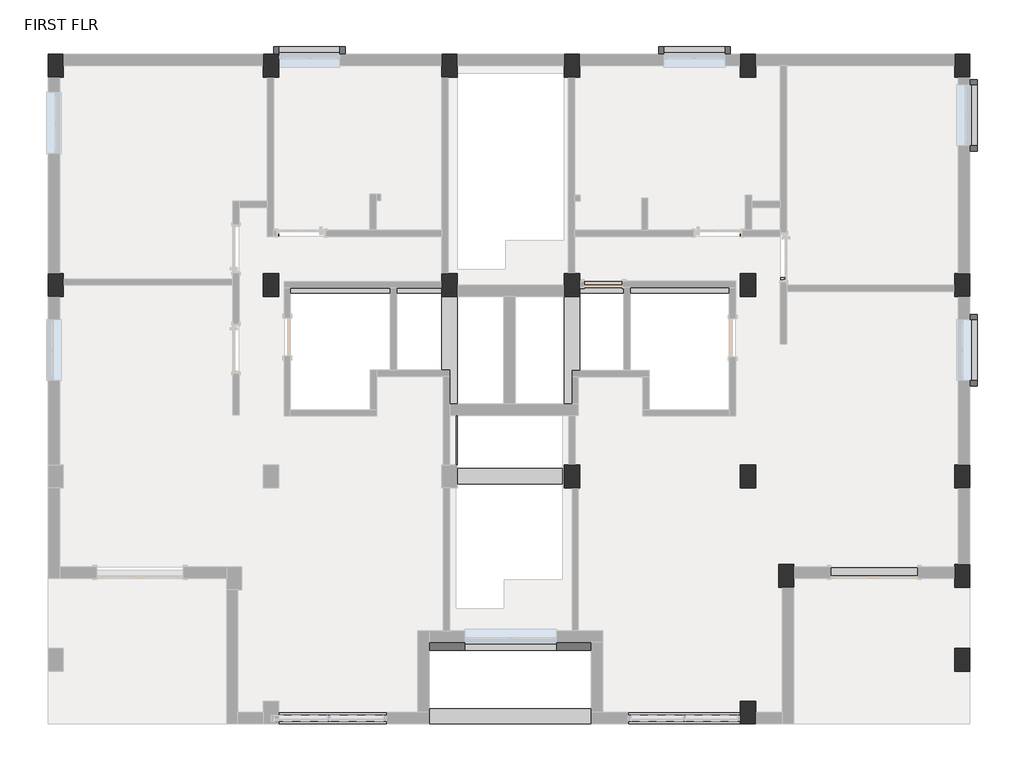
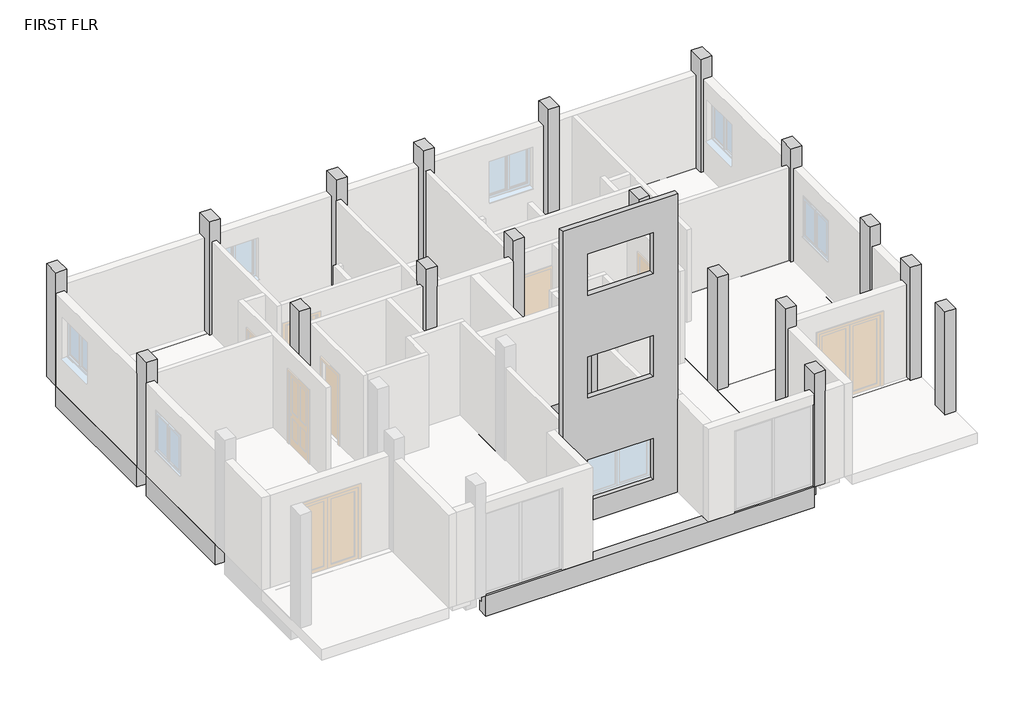
# One storey, part 3 of 3: 31 beams, 19 columns, 5 proxies, 1 light fixture.
"""IFC4 building model written with IfcOpenShell, lengths in millimetres."""

from ifc_helpers import new_model, si_unit, frame, origin, place, context, project, spatial, polyline, outline, extrude, faceted_brep, transform, mapped, element, save
from components import generic_models_10_generic_models_5_40bb8100, generic_models_13_generic_models_13_6edbfaa0, generic_models_2_generic_models_2_e2b5cfd4, column_11789f6a, family2_family2_8c2629c1

model = new_model("IFC4")

# Units and contexts
model_context = context("Model", 3, world=origin())
ifc_project = project(units=[si_unit("LENGTHUNIT", "METRE", prefix="MILLI")], contexts=[model_context])

# Site, building, storey
site = spatial("IfcSite", under=ifc_project)
building = spatial("IfcBuilding", under=site)
storey = spatial("IfcBuildingStorey", under=building, Name="FIRST FLR", Elevation=3352.8)

# Beams
placement = place(None, origin())
element("IfcBeam", 1, ObjectType="Concrete-Rectangular Beam : 12 x 24", at=placement, inside=storey, context=model_context, shape_type="SweptSolid", body=[
    extrude(outline(polyline([(-8839.9786397, -1604.6061634), (-8839.9786397, -1299.8061634), (-4852.9175798, -1299.8061634), (-4852.9175798, -1604.6061634), (-8839.9786397, -1604.6061634)])), frame((0.0, 0.0, 2743.2), z_axis=(0.0, 0.0, 1.0), x_axis=(1.0, 0.0, 0.0)), (0.0, 0.0, 1.0), 609.6),
])
element("IfcBeam", 2, ObjectType="Concrete-Rectangular Beam : 12 x 24", at=placement, inside=storey, context=model_context, shape_type="SweptSolid", body=[
    extrude(outline(polyline([(-1296.9175798, -1299.8061634), (-1296.9175798, -1604.6061634), (-4548.1175798, -1604.6061634), (-4548.1175798, -1299.8061634), (-1296.9175798, -1299.8061634)])), frame((0.0, 0.0, 2743.2), z_axis=(0.0, 0.0, 1.0), x_axis=(1.0, 0.0, 0.0)), (0.0, 0.0, 1.0), 609.6),
])
element("IfcBeam", 3, ObjectType="Concrete-Rectangular Beam : 12 x 24", at=placement, inside=storey, context=model_context, shape_type="SweptSolid", body=[
    extrude(outline(polyline([(1141.4824202, -1299.8061634), (1141.4824202, -1604.6061634), (-992.1175798, -1604.6061634), (-992.1175798, -1299.8061634), (1141.4824202, -1299.8061634)])), frame((0.0, 0.0, 2743.2), z_axis=(0.0, 0.0, 1.0), x_axis=(1.0, 0.0, 0.0)), (0.0, 0.0, 1.0), 609.6),
])
element("IfcBeam", 4, ObjectType="Concrete-Rectangular Beam : 12 x 24", at=placement, inside=storey, context=model_context, shape_type="SweptSolid", body=[
    extrude(outline(polyline([(4646.6824202, -1299.8061634), (4646.6824202, -1604.6061634), (1446.2824202, -1604.6061634), (1446.2824202, -1299.8061634), (4646.6824202, -1299.8061634)])), frame((0.0, 0.0, 2743.2), z_axis=(0.0, 0.0, 1.0), x_axis=(1.0, 0.0, 0.0)), (0.0, 0.0, 1.0), 609.6),
])
element("IfcBeam", 5, ObjectType="Concrete-Rectangular Beam : 12 x 24", at=placement, inside=storey, context=model_context, shape_type="SweptSolid", body=[
    extrude(outline(polyline([(8913.9345022, -1299.8061634), (8913.9345022, -1604.6061634), (4951.5345022, -1604.6061634), (4951.5345022, -1299.8061634), (8913.9345022, -1299.8061634)])), frame((0.0, 0.0, 2743.2), z_axis=(0.0, 0.0, 1.0), x_axis=(1.0, 0.0, 0.0)), (0.0, 0.0, 1.0), 609.6),
])
element("IfcBeam", 6, ObjectType="Concrete-Rectangular Beam : 12 x 24", at=placement, inside=storey, context=model_context, shape_type="SweptSolid", body=[
    extrude(outline(polyline([(9218.6824202, -5600.6620333), (8913.8824202, -5600.6620333), (8913.8824202, -1680.8061634), (9218.6824202, -1680.8061634), (9218.6824202, -5600.6620333)])), frame((0.0, 0.0, 2743.2), z_axis=(0.0, 0.0, 1.0), x_axis=(1.0, 0.0, 0.0)), (0.0, 0.0, 1.0), 609.6),
])
element("IfcBeam", 7, ObjectType="Concrete-Rectangular Beam : 12 x 24", at=placement, inside=storey, context=model_context, shape_type="SweptSolid", body=[
    extrude(outline(polyline([(9218.6824202, -9410.6620333), (8913.8824202, -9410.6620333), (8913.8824202, -6057.8620333), (9218.6824202, -6057.8620333), (9218.6824202, -9410.6620333)])), frame((0.0, 0.0, 2743.2), z_axis=(0.0, 0.0, 1.0), x_axis=(1.0, 0.0, 0.0)), (0.0, 0.0, 1.0), 609.6),
])
element("IfcBeam", 8, ObjectType="Concrete-Rectangular Beam : 12 x 24", at=placement, inside=storey, context=model_context, shape_type="SweptSolid", body=[
    extrude(outline(polyline([(9218.6824202, -11391.8620333), (8913.8824202, -11391.8620333), (8913.8824202, -9867.8620333), (9218.6824202, -9867.8620333), (9218.6824202, -11391.8620333)])), frame((0.0, 0.0, 2743.2), z_axis=(0.0, 0.0, 1.0), x_axis=(1.0, 0.0, 0.0)), (0.0, 0.0, 1.0), 609.6),
])
element("IfcBeam", 9, ObjectType="Concrete-Rectangular Beam : 12 x 24", at=placement, inside=storey, context=model_context, shape_type="SweptSolid", body=[
    extrude(outline(polyline([(-8839.9786397, -5600.6620333), (-9144.7786397, -5600.6620333), (-9144.7786397, -1680.8061634), (-8839.9786397, -1680.8061634), (-8839.9786397, -5600.6620333)])), frame((0.0, 0.0, 2743.2), z_axis=(0.0, 0.0, 1.0), x_axis=(1.0, 0.0, 0.0)), (0.0, 0.0, 1.0), 609.6),
])
element("IfcBeam", 10, ObjectType="Concrete-Rectangular Beam : 12 x 24", at=placement, inside=storey, context=model_context, shape_type="SweptSolid", body=[
    extrude(outline(polyline([(-8839.9786397, -9410.6620333), (-9144.7786397, -9410.6620333), (-9144.7786397, -6057.8620333), (-8839.9786397, -6057.8620333), (-8839.9786397, -9410.6620333)])), frame((0.0, 0.0, 2743.2), z_axis=(0.0, 0.0, 1.0), x_axis=(1.0, 0.0, 0.0)), (0.0, 0.0, 1.0), 609.6),
])
element("IfcBeam", 11, ObjectType="Concrete-Rectangular Beam : 12 x 24", at=placement, inside=storey, context=model_context, shape_type="SweptSolid", body=[
    extrude(outline(polyline([(4951.4824202, -5981.6620333), (4951.4824202, -5676.8620333), (8913.8824202, -5676.8620333), (8913.8824202, -5981.6620333), (4951.4824202, -5981.6620333)])), frame((0.0, 0.0, 2743.2), z_axis=(0.0, 0.0, 1.0), x_axis=(1.0, 0.0, 0.0)), (0.0, 0.0, 1.0), 609.6),
])
element("IfcBeam", 12, ObjectType="Concrete-Rectangular Beam : 12 x 24", at=placement, inside=storey, context=model_context, shape_type="SweptSolid", body=[
    extrude(outline(polyline([(1446.2824202, -5981.6620333), (1446.2824202, -5676.8620333), (4646.6824202, -5676.8620333), (4646.6824202, -5981.6620333), (1446.2824202, -5981.6620333)])), frame((0.0, 0.0, 2743.2), z_axis=(0.0, 0.0, 1.0), x_axis=(1.0, 0.0, 0.0)), (0.0, 0.0, 1.0), 609.6),
])
element("IfcBeam", 13, ObjectType="Concrete-Rectangular Beam : 12 x 24", at=placement, inside=storey, context=model_context, shape_type="SweptSolid", body=[
    extrude(outline(polyline([(-992.1175798, -5981.6620333), (-992.1175798, -5676.8620333), (1141.4824202, -5676.8620333), (1141.4824202, -5981.6620333), (-992.1175798, -5981.6620333)])), frame((0.0, 0.0, 2743.2), z_axis=(0.0, 0.0, 1.0), x_axis=(1.0, 0.0, 0.0)), (0.0, 0.0, 1.0), 609.6),
])
element("IfcBeam", 14, ObjectType="Concrete-Rectangular Beam : 12 x 24", at=placement, inside=storey, context=model_context, shape_type="SweptSolid", body=[
    extrude(outline(polyline([(-4548.1175798, -5981.6620333), (-4548.1175798, -5676.8620333), (-1296.9175798, -5676.8620333), (-1296.9175798, -5981.6620333), (-4548.1175798, -5981.6620333)])), frame((0.0, 0.0, 2743.2), z_axis=(0.0, 0.0, 1.0), x_axis=(1.0, 0.0, 0.0)), (0.0, 0.0, 1.0), 609.6),
])
element("IfcBeam", 15, ObjectType="Concrete-Rectangular Beam : 12 x 24", at=placement, inside=storey, context=model_context, shape_type="SweptSolid", body=[
    extrude(outline(polyline([(-8839.9786397, -5981.6620333), (-8839.9786397, -5676.8620333), (-4852.9175798, -5676.8620333), (-4852.9175798, -5981.6620333), (-8839.9786397, -5981.6620333)])), frame((0.0, 0.0, 2743.2), z_axis=(0.0, 0.0, 1.0), x_axis=(1.0, 0.0, 0.0)), (0.0, 0.0, 1.0), 609.6),
])
element("IfcBeam", 16, ObjectType="Concrete-Rectangular Beam : 12 x 24", at=placement, inside=storey, context=model_context, shape_type="SweptSolid", body=[
    extrude(outline(polyline([(1446.2824202, -9791.6620333), (1446.2824202, -9486.8620333), (4646.6824202, -9486.8620333), (4646.6824202, -9791.6620333), (1446.2824202, -9791.6620333)])), frame((0.0, 0.0, 2743.2), z_axis=(0.0, 0.0, 1.0), x_axis=(1.0, 0.0, 0.0)), (0.0, 0.0, 1.0), 609.6),
])
element("IfcBeam", 17, ObjectType="Concrete-Rectangular Beam : 12 x 24", at=placement, inside=storey, context=model_context, shape_type="Brep", body=[
    faceted_brep([(4951.4824202, -9867.8620333, 3352.8), (4646.6824202, -9867.8620333, 3352.8), (4646.6824202, -11772.8620333, 3352.8), (4951.4824202, -11772.8620333, 3352.8), (4951.4824202, -11468.0620333, 3352.8), (4646.6824202, -9867.8620333, 2743.2), (4646.6824202, -11772.8620333, 2743.2), (4951.4824202, -9867.8620333, 2743.2), (4951.4824202, -11468.0620333, 2743.2), (4951.4824202, -11772.8620333, 2743.2)], [[[0, 1, 2, 3, 4]], [[1, 5, 6, 2]], [[5, 7, 8, 9, 6]], [[7, 0, 4, 3, 9, 8]], [[0, 7, 5, 1]], [[3, 2, 6, 9]]]),
])
element("IfcBeam", 18, ObjectType="Concrete-Rectangular Beam : 12 x 24", at=placement, inside=storey, context=model_context, shape_type="SweptSolid", body=[
    extrude(outline(polyline([(5408.6824202, -11468.0620333), (5408.6824202, -11772.8620333), (4951.4824202, -11772.8620333), (4951.4824202, -11468.0620333), (5408.6824202, -11468.0620333)])), frame((0.0, 0.0, 2743.2), z_axis=(0.0, 0.0, 1.0), x_axis=(1.0, 0.0, 0.0)), (0.0, 0.0, 1.0), 609.6),
])
element("IfcBeam", 19, ObjectType="Concrete-Rectangular Beam : 12 x 24", at=placement, inside=storey, context=model_context, shape_type="SweptSolid", body=[
    extrude(outline(polyline([(8913.8824202, -11468.0620333), (8913.8824202, -11772.8620333), (5713.4824202, -11772.8620333), (5713.4824202, -11468.0620333), (8913.8824202, -11468.0620333)])), frame((0.0, 0.0, 2743.2), z_axis=(0.0, 0.0, 1.0), x_axis=(1.0, 0.0, 0.0)), (0.0, 0.0, 1.0), 609.6),
])
element("IfcBeam", 20, ObjectType="Concrete-Rectangular Beam : 12 x 24", at=placement, inside=storey, context=model_context, shape_type="SweptSolid", body=[
    extrude(outline(polyline([(4646.6824202, -14272.0402089), (4646.6824202, -14576.8402089), (-4548.1175798, -14576.8402089), (-4548.1175798, -14272.0402089), (4646.6824202, -14272.0402089)])), frame((0.0, 0.0, 2743.2), z_axis=(0.0, 0.0, 1.0), x_axis=(1.0, 0.0, 0.0)), (0.0, 0.0, 1.0), 609.6),
])
element("IfcBeam", 21, ObjectType="Concrete-Rectangular Beam : 12 x 24", at=placement, inside=storey, context=model_context, shape_type="SweptSolid", body=[
    extrude(outline(polyline([(4951.4824202, -14119.6402089), (4646.6824202, -14119.6402089), (4646.6824202, -11772.8620333), (4951.4824202, -11772.8620333), (4951.4824202, -14119.6402089)])), frame((0.0, 0.0, 2743.2), z_axis=(0.0, 0.0, 1.0), x_axis=(1.0, 0.0, 0.0)), (0.0, 0.0, 1.0), 609.6),
])
element("IfcBeam", 22, ObjectType="Concrete-Rectangular Beam : 12 x 24", at=placement, inside=storey, context=model_context, shape_type="SweptSolid", body=[
    extrude(outline(polyline([(-4548.1175798, -5600.6620333), (-4852.9175798, -5600.6620333), (-4852.9175798, -1680.8061634), (-4548.1175798, -1680.8061634), (-4548.1175798, -5600.6620333)])), frame((0.0, 0.0, 2743.2), z_axis=(0.0, 0.0, 1.0), x_axis=(1.0, 0.0, 0.0)), (0.0, 0.0, 1.0), 609.6),
])
element("IfcBeam", 23, ObjectType="Concrete-Rectangular Beam : 12 x 24", at=placement, inside=storey, context=model_context, shape_type="SweptSolid", body=[
    extrude(outline(polyline([(-4548.1175798, -9410.6620333), (-4852.9175798, -9410.6620333), (-4852.9175798, -6057.8620333), (-4548.1175798, -6057.8620333), (-4548.1175798, -9410.6620333)])), frame((0.0, 0.0, 2743.2), z_axis=(0.0, 0.0, 1.0), x_axis=(1.0, 0.0, 0.0)), (0.0, 0.0, 1.0), 609.6),
])
element("IfcBeam", 24, ObjectType="Concrete-Rectangular Beam : 12 x 24", at=placement, inside=storey, context=model_context, shape_type="SweptSolid", body=[
    extrude(outline(polyline([(-992.1175798, -5600.6620333), (-1296.9175798, -5600.6620333), (-1296.9175798, -1680.8061634), (-992.1175798, -1680.8061634), (-992.1175798, -5600.6620333)])), frame((0.0, 0.0, 2743.2), z_axis=(0.0, 0.0, 1.0), x_axis=(1.0, 0.0, 0.0)), (0.0, 0.0, 1.0), 609.6),
])
element("IfcBeam", 25, ObjectType="Concrete-Rectangular Beam : 12 x 24", at=placement, inside=storey, context=model_context, shape_type="SweptSolid", body=[
    extrude(outline(polyline([(-992.1175798, -9410.6620333), (-1296.9175798, -9410.6620333), (-1296.9175798, -6057.8620333), (-992.1175798, -6057.8620333), (-992.1175798, -9410.6620333)])), frame((0.0, 0.0, 2743.2), z_axis=(0.0, 0.0, 1.0), x_axis=(1.0, 0.0, 0.0)), (0.0, 0.0, 1.0), 609.6),
])
element("IfcBeam", 26, ObjectType="Concrete-Rectangular Beam : 12 x 24", at=placement, inside=storey, context=model_context, shape_type="SweptSolid", body=[
    extrude(outline(polyline([(1141.4824202, -6057.8620333), (1446.2824202, -6057.8620333), (1446.2824202, -9410.6620333), (1141.4824202, -9410.6620333), (1141.4824202, -6057.8620333)])), frame((0.0, 0.0, 2743.2), z_axis=(0.0, 0.0, 1.0), x_axis=(1.0, 0.0, 0.0)), (0.0, 0.0, 1.0), 609.6),
])
element("IfcBeam", 27, ObjectType="Concrete-Rectangular Beam : 12 x 24", at=placement, inside=storey, context=model_context, shape_type="SweptSolid", body=[
    extrude(outline(polyline([(1141.4824202, -1680.8061634), (1446.2824202, -1680.8061634), (1446.2824202, -5600.6620333), (1141.4824202, -5600.6620333), (1141.4824202, -1680.8061634)])), frame((0.0, 0.0, 2743.2), z_axis=(0.0, 0.0, 1.0), x_axis=(1.0, 0.0, 0.0)), (0.0, 0.0, 1.0), 609.6),
])
element("IfcBeam", 28, ObjectType="Concrete-Rectangular Beam : 12 x 24", at=placement, inside=storey, context=model_context, shape_type="SweptSolid", body=[
    extrude(outline(polyline([(4951.4824202, -5600.6620333), (4646.6824202, -5600.6620333), (4646.6824202, -1680.8061634), (4951.4824202, -1680.8061634), (4951.4824202, -5600.6620333)])), frame((0.0, 0.0, 2743.2), z_axis=(0.0, 0.0, 1.0), x_axis=(1.0, 0.0, 0.0)), (0.0, 0.0, 1.0), 609.6),
])
element("IfcBeam", 29, ObjectType="Concrete-Rectangular Beam : 12 x 24", at=placement, inside=storey, context=model_context, shape_type="SweptSolid", body=[
    extrude(outline(polyline([(4951.4824202, -9410.6620333), (4646.6824202, -9410.6620333), (4646.6824202, -6057.8620333), (4951.4824202, -6057.8620333), (4951.4824202, -9410.6620333)])), frame((0.0, 0.0, 2743.2), z_axis=(0.0, 0.0, 1.0), x_axis=(1.0, 0.0, 0.0)), (0.0, 0.0, 1.0), 609.6),
])
element("IfcBeam", 30, ObjectType="Concrete-Rectangular Beam : 12 x 24", at=placement, inside=storey, context=model_context, shape_type="SweptSolid", body=[
    extrude(outline(polyline([(4951.4824202, -9791.6620333), (4951.4824202, -9486.8620333), (8913.8824202, -9486.8620333), (8913.8824202, -9791.6620333), (4951.4824202, -9791.6620333)])), frame((0.0, 0.0, 2743.2), z_axis=(0.0, 0.0, 1.0), x_axis=(1.0, 0.0, 0.0)), (0.0, 0.0, 1.0), 609.6),
])
element("IfcBeam", 31, ObjectType="Concrete-Rectangular Beam : 12 x 24", at=placement, inside=storey, context=model_context, shape_type="SweptSolid", body=[
    extrude(outline(polyline([(1141.4824202, -9486.8620333), (1141.4824202, -9791.6620333), (-992.1175798, -9791.6620333), (-992.1175798, -9486.8620333), (1141.4824202, -9486.8620333)])), frame((0.0, 0.0, 2743.2), z_axis=(0.0, 0.0, 1.0), x_axis=(1.0, 0.0, 0.0)), (0.0, 0.0, 1.0), 609.6),
])

# Proxies
generic_models_10_generic_models_5_shape = generic_models_10_generic_models_5_40bb8100(model_context)
element("IfcBuildingElementProxy", 32, Name="Generic Models 11 : Generic Models 5", ObjectType="Generic Models 11 : Generic Models 5", at=placement, inside=storey, context=model_context, shape_type="MappedRepresentation", body=[
    mapped(generic_models_10_generic_models_5_shape, transform((0.0, 0.0, -6096.0), x_axis=(1.0, 0.0, 0.0), y_axis=(0.0, 1.0, 0.0), z_axis=(0.0, 0.0, 1.0))),
])
generic_models_13_generic_models_13_shape = generic_models_13_generic_models_13_6edbfaa0(model_context)
element("IfcBuildingElementProxy", 33, Name="Generic Models 16 : Generic Models 13", ObjectType="Generic Models 16 : Generic Models 13", at=placement, inside=storey, context=model_context, shape_type="MappedRepresentation", body=[
    mapped(generic_models_13_generic_models_13_shape, transform((0.0, 0.0, -6096.0), x_axis=(1.0, 0.0, 0.0), y_axis=(0.0, 1.0, 0.0), z_axis=(0.0, 0.0, 1.0))),
])
element("IfcBuildingElementProxy", 34, Name="Generic Models 17 : Generic Models 13", ObjectType="Generic Models 17 : Generic Models 13", at=placement, inside=storey, context=model_context, shape_type="MappedRepresentation", body=[
    mapped(generic_models_13_generic_models_13_shape, transform((-7670.8, 0.0, -6096.0), x_axis=(1.0, 0.0, 0.0), y_axis=(0.0, 1.0, 0.0), z_axis=(0.0, 0.0, 1.0))),
])
generic_models_2_generic_models_2_shape = generic_models_2_generic_models_2_e2b5cfd4(model_context)
element("IfcBuildingElementProxy", 35, Name="Generic Models 2 : Generic Models 2", ObjectType="Generic Models 2 : Generic Models 2", at=placement, inside=storey, context=model_context, shape_type="MappedRepresentation", body=[
    mapped(generic_models_2_generic_models_2_shape, transform((0.0, 0.0, 0.0), x_axis=(1.0, 0.0, 0.0), y_axis=(0.0, 1.0, 0.0), z_axis=(0.0, 0.0, 1.0))),
])
element("IfcBuildingElementProxy", 36, Name="Generic Models 8 : Generic Models 5", ObjectType="Generic Models 8 : Generic Models 5", at=placement, inside=storey, context=model_context, shape_type="MappedRepresentation", body=[
    mapped(generic_models_10_generic_models_5_shape, transform((0.0, 4681.8558699, -6096.0), x_axis=(1.0, 0.0, 0.0), y_axis=(0.0, 1.0, 0.0), z_axis=(0.0, 0.0, 1.0))),
])

# Columns
element("IfcColumn", 37, ObjectType="Concrete-Rectangular-Column : 1'6\" X 1' COLUMN", at=placement, inside=storey, context=model_context, shape_type="Brep", body=[
    faceted_brep([(-8839.9786397, -1223.6061634, 3352.8), (-8839.9786397, -1680.8061634, 3352.8), (-9144.7786397, -1680.8061634, 3352.8), (-9144.7786397, -1223.6061634, 3352.8), (-8839.9786397, -1223.6061634, 6705.6), (-8839.9786397, -1299.8061634, 6705.6), (-8839.9786397, -1604.6061634, 6705.6), (-8839.9786397, -1680.8061634, 6705.6), (-8839.9786397, -1680.8061634, 6096.0), (-8839.9786397, -1680.8061634, 5791.2), (-9144.7786397, -1680.8061634, 6705.6), (-9144.7786397, -1680.8061634, 6096.0), (-9144.7786397, -1680.8061634, 5791.2), (-9144.7786397, -1223.6061634, 6705.6)], [[[0, 1, 2, 3]], [[4, 5, 6, 7, 8, 9, 1, 0]], [[7, 10, 11, 12, 2, 1, 9, 8]], [[10, 13, 3, 2, 12, 11]], [[13, 4, 0, 3]], [[4, 13, 10, 7, 6, 5]]]),
])
element("IfcColumn", 38, ObjectType="Concrete-Rectangular-Column : 1'6\" X 1' COLUMN", at=placement, inside=storey, context=model_context, shape_type="Brep", body=[
    faceted_brep([(-4548.1175798, -1223.6061634, 3352.8), (-4548.1175798, -1680.8061634, 3352.8), (-4852.9175798, -1680.8061634, 3352.8), (-4852.9175798, -1223.6061634, 3352.8), (-4548.1175798, -1223.6061634, 6705.6), (-4548.1175798, -1299.8061634, 6705.6), (-4548.1175798, -1604.6061634, 6705.6), (-4548.1175798, -1680.8061634, 6705.6), (-4548.1175798, -1680.8061634, 6096.0), (-4548.1175798, -1680.8061634, 5791.2), (-4852.9175798, -1680.8061634, 6705.6), (-4852.9175798, -1680.8061634, 6096.0), (-4852.9175798, -1680.8061634, 5791.2), (-4852.9175798, -1223.6061634, 6705.6)], [[[0, 1, 2, 3]], [[4, 5, 6, 7, 8, 9, 1, 0]], [[7, 10, 11, 12, 2, 1, 9, 8]], [[10, 13, 3, 2, 12, 11]], [[13, 4, 0, 3]], [[4, 13, 10, 7, 6, 5]]]),
])
element("IfcColumn", 39, ObjectType="Concrete-Rectangular-Column : 1'6\" X 1' COLUMN", at=placement, inside=storey, context=model_context, shape_type="Brep", body=[
    faceted_brep([(-992.1175798, -1223.6061634, 3352.8), (-992.1175798, -1680.8061634, 3352.8), (-1296.9175798, -1680.8061634, 3352.8), (-1296.9175798, -1223.6061634, 3352.8), (-992.1175798, -1223.6061634, 6705.6), (-992.1175798, -1299.8061634, 6705.6), (-992.1175798, -1604.6061634, 6705.6), (-992.1175798, -1680.8061634, 6705.6), (-992.1175798, -1680.8061634, 6096.0), (-992.1175798, -1680.8061634, 5791.2), (-1296.9175798, -1680.8061634, 6705.6), (-1296.9175798, -1680.8061634, 6096.0), (-1296.9175798, -1680.8061634, 5791.2), (-1296.9175798, -1604.6061634, 6705.6), (-1296.9175798, -1299.8061634, 6705.6), (-1296.9175798, -1223.6061634, 6705.6)], [[[0, 1, 2, 3]], [[4, 5, 6, 7, 8, 9, 1, 0]], [[7, 10, 11, 12, 2, 1, 9, 8]], [[10, 13, 14, 15, 3, 2, 12, 11]], [[15, 4, 0, 3]], [[4, 15, 14, 13, 10, 7, 6, 5]]]),
])
element("IfcColumn", 40, ObjectType="Concrete-Rectangular-Column : 1'6\" X 1' COLUMN", at=placement, inside=storey, context=model_context, shape_type="Brep", body=[
    faceted_brep([(1446.2824202, -1223.6061634, 3352.8), (1446.2824202, -1680.8061634, 3352.8), (1141.4824202, -1680.8061634, 3352.8), (1141.4824202, -1223.6061634, 3352.8), (1446.2824202, -1223.6061634, 6705.6), (1446.2824202, -1299.8061634, 6705.6), (1446.2824202, -1604.6061634, 6705.6), (1446.2824202, -1680.8061634, 6705.6), (1446.2824202, -1680.8061634, 6096.0), (1446.2824202, -1680.8061634, 5791.2), (1141.4824202, -1680.8061634, 6705.6), (1141.4824202, -1680.8061634, 6096.0), (1141.4824202, -1680.8061634, 5791.2), (1141.4824202, -1604.6061634, 6705.6), (1141.4824202, -1299.8061634, 6705.6), (1141.4824202, -1223.6061634, 6705.6)], [[[0, 1, 2, 3]], [[4, 5, 6, 7, 8, 9, 1, 0]], [[7, 10, 11, 12, 2, 1, 9, 8]], [[10, 13, 14, 15, 3, 2, 12, 11]], [[15, 4, 0, 3]], [[4, 15, 14, 13, 10, 7, 6, 5]]]),
])
element("IfcColumn", 41, ObjectType="Concrete-Rectangular-Column : 1'6\" X 1' COLUMN", at=placement, inside=storey, context=model_context, shape_type="Brep", body=[
    faceted_brep([(4951.4824202, -1223.6061634, 3352.8), (4951.4824202, -1680.8061634, 3352.8), (4646.6824202, -1680.8061634, 3352.8), (4646.6824202, -1223.6061634, 3352.8), (4951.4824202, -1223.6061634, 6705.6), (4951.4824202, -1680.8061634, 6705.6), (4951.4824202, -1680.8061634, 6096.0), (4951.4824202, -1680.8061634, 5791.2), (4646.6824202, -1680.8061634, 6705.6), (4646.6824202, -1680.8061634, 6096.0), (4646.6824202, -1680.8061634, 5791.2), (4646.6824202, -1604.6061634, 6705.6), (4646.6824202, -1299.8061634, 6705.6), (4646.6824202, -1223.6061634, 6705.6)], [[[0, 1, 2, 3]], [[4, 5, 6, 7, 1, 0]], [[5, 8, 9, 10, 2, 1, 7, 6]], [[8, 11, 12, 13, 3, 2, 10, 9]], [[13, 4, 0, 3]], [[4, 13, 12, 11, 8, 5]]]),
])
element("IfcColumn", 42, ObjectType="Concrete-Rectangular-Column : 1'6\" X 1' COLUMN", at=placement, inside=storey, context=model_context, shape_type="Brep", body=[
    faceted_brep([(9218.6824202, -1223.6061634, 3352.8), (9218.6824202, -1680.8061634, 3352.8), (8913.8824202, -1680.8061634, 3352.8), (8913.8824202, -1223.6061634, 3352.8), (9218.6824202, -1223.6061634, 6705.6), (9218.6824202, -1680.8061634, 6705.6), (9218.6824202, -1680.8061634, 6096.0), (9218.6824202, -1680.8061634, 5791.2), (8913.8824202, -1680.8061634, 6705.6), (8913.8824202, -1680.8061634, 6096.0), (8913.8824202, -1680.8061634, 5791.2), (8913.8824202, -1223.6061634, 6705.6)], [[[0, 1, 2, 3]], [[4, 5, 6, 7, 1, 0]], [[5, 8, 9, 10, 2, 1, 7, 6]], [[8, 11, 3, 2, 10, 9]], [[11, 4, 0, 3]], [[4, 11, 8, 5]]]),
])
element("IfcColumn", 43, ObjectType="Concrete-Rectangular-Column : 1'6\" X 1' COLUMN", at=placement, inside=storey, context=model_context, shape_type="Brep", body=[
    faceted_brep([(9218.6824202, -5600.6620333, 3352.8), (9218.6824202, -6057.8620333, 3352.8), (8913.8824202, -6057.8620333, 3352.8), (8913.8824202, -5600.6620333, 3352.8), (9218.6824202, -5600.6620333, 6705.6), (9218.6824202, -6057.8620333, 6705.6), (9218.6824202, -6057.8620333, 6096.0), (9218.6824202, -6057.8620333, 5791.2), (9218.6824202, -5600.6620333, 5791.2), (9218.6824202, -5600.6620333, 6096.0), (8913.8824202, -6057.8620333, 6705.6), (8913.8824202, -6057.8620333, 6096.0), (8913.8824202, -6057.8620333, 5791.2), (8913.8824202, -5981.6620333, 6705.6), (8913.8824202, -5676.8620333, 6705.6), (8913.8824202, -5600.6620333, 6705.6), (8913.8824202, -5600.6620333, 6096.0), (8913.8824202, -5600.6620333, 5791.2)], [[[0, 1, 2, 3]], [[4, 5, 6, 7, 1, 0, 8, 9]], [[5, 10, 11, 12, 2, 1, 7, 6]], [[10, 13, 14, 15, 16, 17, 3, 2, 12, 11]], [[15, 4, 9, 8, 0, 3, 17, 16]], [[4, 15, 14, 13, 10, 5]]]),
])
element("IfcColumn", 44, ObjectType="Concrete-Rectangular-Column : 1'6\" X 1' COLUMN", at=placement, inside=storey, context=model_context, shape_type="Brep", body=[
    faceted_brep([(4951.4824202, -5600.6620333, 3352.8), (4951.4824202, -6057.8620333, 3352.8), (4646.6824202, -6057.8620333, 3352.8), (4646.6824202, -5600.6620333, 3352.8), (4951.4824202, -5600.6620333, 6705.6), (4951.4824202, -5676.8620333, 6705.6), (4951.4824202, -5981.6620333, 6705.6), (4951.4824202, -6057.8620333, 6705.6), (4951.4824202, -6057.8620333, 6096.0), (4951.4824202, -6057.8620333, 5791.2), (4951.4824202, -5600.6620333, 5791.2), (4951.4824202, -5600.6620333, 6096.0), (4646.6824202, -6057.8620333, 6705.6), (4646.6824202, -6057.8620333, 6096.0), (4646.6824202, -6057.8620333, 5791.2), (4646.6824202, -5981.6620333, 6705.6), (4646.6824202, -5676.8620333, 6705.6), (4646.6824202, -5600.6620333, 6705.6), (4646.6824202, -5600.6620333, 6096.0), (4646.6824202, -5600.6620333, 5791.2)], [[[0, 1, 2, 3]], [[4, 5, 6, 7, 8, 9, 1, 0, 10, 11]], [[7, 12, 13, 14, 2, 1, 9, 8]], [[12, 15, 16, 17, 18, 19, 3, 2, 14, 13]], [[17, 4, 11, 10, 0, 3, 19, 18]], [[4, 17, 16, 15, 12, 7, 6, 5]]]),
])
element("IfcColumn", 45, ObjectType="Concrete-Rectangular-Column : 1'6\" X 1' COLUMN", at=placement, inside=storey, context=model_context, shape_type="Brep", body=[
    faceted_brep([(1446.2824202, -5600.6620333, 3352.8), (1446.2824202, -6057.8620333, 3352.8), (1141.4824202, -6057.8620333, 3352.8), (1141.4824202, -5600.6620333, 3352.8), (1446.2824202, -5600.6620333, 6705.6), (1446.2824202, -5676.8620333, 6705.6), (1446.2824202, -5981.6620333, 6705.6), (1446.2824202, -6057.8620333, 6705.6), (1446.2824202, -6057.8620333, 6096.0), (1446.2824202, -6057.8620333, 5791.2), (1446.2824202, -5600.6620333, 5791.2), (1446.2824202, -5600.6620333, 6096.0), (1141.4824202, -6057.8620333, 6705.6), (1141.4824202, -6057.8620333, 6096.0), (1141.4824202, -6057.8620333, 5791.2), (1141.4824202, -5981.6620333, 6705.6), (1141.4824202, -5676.8620333, 6705.6), (1141.4824202, -5600.6620333, 6705.6), (1141.4824202, -5600.6620333, 6096.0), (1141.4824202, -5600.6620333, 5791.2)], [[[0, 1, 2, 3]], [[4, 5, 6, 7, 8, 9, 1, 0, 10, 11]], [[7, 12, 13, 14, 2, 1, 9, 8]], [[12, 15, 16, 17, 18, 19, 3, 2, 14, 13]], [[17, 4, 11, 10, 0, 3, 19, 18]], [[4, 17, 16, 15, 12, 7, 6, 5]]]),
])
element("IfcColumn", 46, ObjectType="Concrete-Rectangular-Column : 1'6\" X 1' COLUMN", at=placement, inside=storey, context=model_context, shape_type="Brep", body=[
    faceted_brep([(-992.1175798, -5600.6620333, 3352.8), (-992.1175798, -6057.8620333, 3352.8), (-1296.9175798, -6057.8620333, 3352.8), (-1296.9175798, -5600.6620333, 3352.8), (-992.1175798, -5600.6620333, 6705.6), (-992.1175798, -5676.8620333, 6705.6), (-992.1175798, -5981.6620333, 6705.6), (-992.1175798, -6057.8620333, 6705.6), (-992.1175798, -6057.8620333, 6096.0), (-992.1175798, -6057.8620333, 5791.2), (-992.1175798, -5600.6620333, 5791.2), (-992.1175798, -5600.6620333, 6096.0), (-1296.9175798, -6057.8620333, 6705.6), (-1296.9175798, -6057.8620333, 6096.0), (-1296.9175798, -6057.8620333, 5791.2), (-1296.9175798, -5981.6620333, 6705.6), (-1296.9175798, -5676.8620333, 6705.6), (-1296.9175798, -5600.6620333, 6705.6), (-1296.9175798, -5600.6620333, 6096.0), (-1296.9175798, -5600.6620333, 5791.2)], [[[0, 1, 2, 3]], [[4, 5, 6, 7, 8, 9, 1, 0, 10, 11]], [[7, 12, 13, 14, 2, 1, 9, 8]], [[12, 15, 16, 17, 18, 19, 3, 2, 14, 13]], [[17, 4, 11, 10, 0, 3, 19, 18]], [[4, 17, 16, 15, 12, 7, 6, 5]]]),
])
element("IfcColumn", 47, ObjectType="Concrete-Rectangular-Column : 1'6\" X 1' COLUMN", at=placement, inside=storey, context=model_context, shape_type="Brep", body=[
    faceted_brep([(-4548.1175798, -5600.6620333, 3352.8), (-4548.1175798, -6057.8620333, 3352.8), (-4852.9175798, -6057.8620333, 3352.8), (-4852.9175798, -5600.6620333, 3352.8), (-4548.1175798, -5600.6620333, 6705.6), (-4548.1175798, -5676.8620333, 6705.6), (-4548.1175798, -5981.6620333, 6705.6), (-4548.1175798, -6057.8620333, 6705.6), (-4548.1175798, -6057.8620333, 6096.0), (-4548.1175798, -6057.8620333, 5791.2), (-4548.1175798, -5600.6620333, 5791.2), (-4548.1175798, -5600.6620333, 6096.0), (-4852.9175798, -6057.8620333, 6705.6), (-4852.9175798, -6057.8620333, 6096.0), (-4852.9175798, -6057.8620333, 5791.2), (-4852.9175798, -5981.6620333, 6705.6), (-4852.9175798, -5676.8620333, 6705.6), (-4852.9175798, -5600.6620333, 6705.6), (-4852.9175798, -5600.6620333, 6096.0), (-4852.9175798, -5600.6620333, 5791.2)], [[[0, 1, 2, 3]], [[4, 5, 6, 7, 8, 9, 1, 0, 10, 11]], [[7, 12, 13, 14, 2, 1, 9, 8]], [[12, 15, 16, 17, 18, 19, 3, 2, 14, 13]], [[17, 4, 11, 10, 0, 3, 19, 18]], [[4, 17, 16, 15, 12, 7, 6, 5]]]),
])
element("IfcColumn", 48, ObjectType="Concrete-Rectangular-Column : 1'6\" X 1' COLUMN", at=placement, inside=storey, context=model_context, shape_type="Brep", body=[
    faceted_brep([(-8839.9786397, -5600.6620333, 3352.8), (-8839.9786397, -6057.8620333, 3352.8), (-9144.7786397, -6057.8620333, 3352.8), (-9144.7786397, -5600.6620333, 3352.8), (-8839.9786397, -5600.6620333, 6705.6), (-8839.9786397, -5676.8620333, 6705.6), (-8839.9786397, -5981.6620333, 6705.6), (-8839.9786397, -6057.8620333, 6705.6), (-8839.9786397, -6057.8620333, 6096.0), (-8839.9786397, -6057.8620333, 5791.2), (-8839.9786397, -5600.6620333, 5791.2), (-8839.9786397, -5600.6620333, 6096.0), (-9144.7786397, -6057.8620333, 6705.6), (-9144.7786397, -6057.8620333, 6096.0), (-9144.7786397, -6057.8620333, 5791.2), (-9144.7786397, -5600.6620333, 6705.6), (-9144.7786397, -5600.6620333, 6096.0), (-9144.7786397, -5600.6620333, 5791.2)], [[[0, 1, 2, 3]], [[4, 5, 6, 7, 8, 9, 1, 0, 10, 11]], [[7, 12, 13, 14, 2, 1, 9, 8]], [[12, 15, 16, 17, 3, 2, 14, 13]], [[15, 4, 11, 10, 0, 3, 17, 16]], [[4, 15, 12, 7, 6, 5]]]),
])
element("IfcColumn", 49, ObjectType="Concrete-Rectangular-Column : 1'6\" X 1' COLUMN", at=placement, inside=storey, context=model_context, shape_type="Brep", body=[
    faceted_brep([(9218.6824202, -11391.8620333, 3352.8), (9218.6824202, -11849.0620333, 3352.8), (8913.8824202, -11849.0620333, 3352.8), (8913.8824202, -11391.8620333, 3352.8), (9218.6824202, -11391.8620333, 6705.6), (9218.6824202, -11849.0620333, 6705.6), (9218.6824202, -11391.8620333, 5791.2), (9218.6824202, -11391.8620333, 6096.0), (8913.8824202, -11849.0620333, 6705.6), (8913.8824202, -11772.8620333, 6705.6), (8913.8824202, -11468.0620333, 6705.6), (8913.8824202, -11391.8620333, 6705.6), (8913.8824202, -11391.8620333, 6096.0), (8913.8824202, -11391.8620333, 5791.2)], [[[0, 1, 2, 3]], [[4, 5, 1, 0, 6, 7]], [[5, 8, 2, 1]], [[8, 9, 10, 11, 12, 13, 3, 2]], [[11, 4, 7, 6, 0, 3, 13, 12]], [[4, 11, 10, 9, 8, 5]]]),
])
element("IfcColumn", 50, ObjectType="Concrete-Rectangular-Column : 1'6\" X 1' COLUMN", at=placement, inside=storey, context=model_context, shape_type="Brep", body=[
    faceted_brep([(9218.6824202, -9410.6620333, 3352.8), (9218.6824202, -9867.8620333, 3352.8), (8913.8824202, -9867.8620333, 3352.8), (8913.8824202, -9410.6620333, 3352.8), (9218.6824202, -9410.6620333, 6705.6), (9218.6824202, -9867.8620333, 6705.6), (9218.6824202, -9867.8620333, 6096.0), (9218.6824202, -9867.8620333, 5791.2), (9218.6824202, -9410.6620333, 5791.2), (9218.6824202, -9410.6620333, 6096.0), (8913.8824202, -9867.8620333, 6705.6), (8913.8824202, -9867.8620333, 6096.0), (8913.8824202, -9867.8620333, 5791.2), (8913.8824202, -9791.6620333, 6705.6), (8913.8824202, -9486.8620333, 6705.6), (8913.8824202, -9410.6620333, 6705.6), (8913.8824202, -9410.6620333, 6096.0), (8913.8824202, -9410.6620333, 5791.2)], [[[0, 1, 2, 3]], [[4, 5, 6, 7, 1, 0, 8, 9]], [[5, 10, 11, 12, 2, 1, 7, 6]], [[10, 13, 14, 15, 16, 17, 3, 2, 12, 11]], [[15, 4, 9, 8, 0, 3, 17, 16]], [[4, 15, 14, 13, 10, 5]]]),
])
element("IfcColumn", 51, ObjectType="Concrete-Rectangular-Column : 1'6\" X 1' COLUMN", at=placement, inside=storey, context=model_context, shape_type="Brep", body=[
    faceted_brep([(4951.4824202, -9410.6620333, 3352.8), (4951.4824202, -9867.8620333, 3352.8), (4646.6824202, -9867.8620333, 3352.8), (4646.6824202, -9410.6620333, 3352.8), (4951.4824202, -9410.6620333, 6705.6), (4951.4824202, -9486.8620333, 6705.6), (4951.4824202, -9791.6620333, 6705.6), (4951.4824202, -9867.8620333, 6705.6), (4951.4824202, -9410.6620333, 5791.2), (4951.4824202, -9410.6620333, 6096.0), (4646.6824202, -9867.8620333, 6705.6), (4646.6824202, -9410.6620333, 6705.6), (4646.6824202, -9410.6620333, 6096.0), (4646.6824202, -9410.6620333, 5791.2)], [[[0, 1, 2, 3]], [[4, 5, 6, 7, 1, 0, 8, 9]], [[7, 10, 2, 1]], [[10, 11, 12, 13, 3, 2]], [[11, 4, 9, 8, 0, 3, 13, 12]], [[4, 11, 10, 7, 6, 5]]]),
])
element("IfcColumn", 52, ObjectType="Concrete-Rectangular-Column : 1'6\" X 1' COLUMN", at=placement, inside=storey, context=model_context, shape_type="Brep", body=[
    faceted_brep([(1446.2824202, -9410.6620333, 3352.8), (1446.2824202, -9867.8620333, 3352.8), (1141.4824202, -9867.8620333, 3352.8), (1141.4824202, -9410.6620333, 3352.8), (1446.2824202, -9410.6620333, 6705.6), (1446.2824202, -9486.8620333, 6705.6), (1446.2824202, -9791.6620333, 6705.6), (1446.2824202, -9867.8620333, 6705.6), (1446.2824202, -9410.6620333, 5791.2), (1446.2824202, -9410.6620333, 6096.0), (1141.4824202, -9867.8620333, 6705.6), (1141.4824202, -9410.6620333, 6705.6), (1141.4824202, -9410.6620333, 6096.0), (1141.4824202, -9410.6620333, 5791.2)], [[[0, 1, 2, 3]], [[4, 5, 6, 7, 1, 0, 8, 9]], [[7, 10, 2, 1]], [[10, 11, 12, 13, 3, 2]], [[11, 4, 9, 8, 0, 3, 13, 12]], [[4, 11, 10, 7, 6, 5]]]),
])
element("IfcColumn", 53, ObjectType="Concrete-Rectangular-Column : 1'6\" X 1' COLUMN", at=placement, inside=storey, context=model_context, shape_type="Brep", body=[
    faceted_brep([(5713.4824202, -11391.8620333, 3352.8), (5713.4824202, -11849.0620333, 3352.8), (5408.6824202, -11849.0620333, 3352.8), (5408.6824202, -11391.8620333, 3352.8), (5713.4824202, -11391.8620333, 6705.6), (5713.4824202, -11468.0620333, 6705.6), (5713.4824202, -11772.8620333, 6705.6), (5713.4824202, -11849.0620333, 6705.6), (5408.6824202, -11849.0620333, 6705.6), (5408.6824202, -11391.8620333, 6705.6)], [[[0, 1, 2, 3]], [[4, 5, 6, 7, 1, 0]], [[7, 8, 2, 1]], [[8, 9, 3, 2]], [[9, 4, 0, 3]], [[4, 9, 8, 7, 6, 5]]]),
])
element("IfcColumn", 54, ObjectType="Concrete-Rectangular-Column : 1'6\" X 1' COLUMN", at=placement, inside=storey, context=model_context, shape_type="Brep", body=[
    faceted_brep([(4951.4824202, -14119.6402089, 3352.8), (4951.4824202, -14576.8402089, 3352.8), (4646.6824202, -14576.8402089, 3352.8), (4646.6824202, -14119.6402089, 3352.8), (4951.4824202, -14119.6402089, 6705.6), (4951.4824202, -14576.8402089, 6705.6), (4646.6824202, -14576.8402089, 6705.6), (4646.6824202, -14576.8402089, 6400.8), (4646.6824202, -14576.8402089, 5791.2), (4646.6824202, -14119.6402089, 6705.6)], [[[0, 1, 2, 3]], [[4, 5, 1, 0]], [[5, 6, 7, 8, 2, 1]], [[6, 9, 3, 2, 8, 7]], [[9, 4, 0, 3]], [[4, 9, 6, 5]]]),
])
column_shape = column_11789f6a(model_context)
element("IfcColumn", 55, ObjectType="Concrete-Rectangular-Column : 1'6\" X 1' COLUMN", at=placement, inside=storey, context=model_context, shape_type="MappedRepresentation", body=[
    mapped(column_shape, transform((9066.2824202, -13294.1402089, 0.0), x_axis=(1.0, 0.0, 0.0), y_axis=(0.0, 1.0, 0.0), z_axis=(0.0, 0.0, 1.0))),
])

# Light fixture
family2_family2_shape = family2_family2_8c2629c1(model_context)
element("IfcLightFixture", 56, ObjectType="Family2 : Family2", at=placement, inside=storey, context=model_context, shape_type="MappedRepresentation", body=[
    mapped(family2_family2_shape, transform((-4903.7175798, -1871.3061634, 101.6), x_axis=(1.0, 0.0, 0.0), y_axis=(0.0, 1.0, 0.0), z_axis=(0.0, 0.0, 1.0))),
])

save(model, "model.ifc")

# Revit data of these elements
# Type "Concrete-Rectangular Beam : 12 x 24"
#   Assembly Code = "B10"
#   Length [instance default] = 5' - 0"
#   b = 1' - 0"
#   h = 2' - 0"
#   Structural Material [instance default] = Concrete, Cast-in-Place gray
# Type "Concrete-Rectangular-Column : 1'6\" X 1' COLUMN"
#   Assembly Code = "B10"
#   b = 1' - 0"
#   h = 1' - 6"
#   Structural Material [instance default] = Concrete, Cast-in-Place gray
# Type "Family2 : Family2"
#   Wattage = 27 W
#   built-in parameter 1150110 = 1 (stored number, unit not read)
#   built-in parameter 1114217 = 1 (stored number, unit not read)
#   built-in parameter 1150109 = 1 (stored number, unit not read)
#   built-in parameter 1150113 = 1 (stored number, unit not read)
#   Lumens = 4010.63 lm
#   built-in parameter 1150115 = 1 (stored number, unit not read)
#   built-in parameter 1150105 = 319.156 (stored number, unit not read)
#   Light Source Symbol Size = 2' - 0"
#   built-in parameter 1150112 = 1 (stored number, unit not read)
#   built-in parameter 1150114 = 1 (stored number, unit not read)
#   built-in parameter 1150107 = 3000 (stored number, unit not read)
#   built-in parameter 1150106 = 3.19156 (stored number, unit not read)
#   built-in parameter 1150104 = 13.8 (stored number, unit not read)
#   built-in parameter 1114218 = 1 (stored number, unit not read)
#   built-in parameter 1150133 = 10 (stored number, unit not read)
#   Color Filter = 16777215
#   Dimming Lamp Color Temperature Shift = (empty or 0)
#   Default Elevation = 0
# Elements 1, 2, 3, 4, 5, 6, 7, 9, 10, 11, 12, 13, 14, 15, 16, 17, 18, 19, 20, 21, 22, 23, 24, 25, 26, 27, 28, 29, 30, 31 (IfcBeam, "Concrete-Rectangular Beam : 12 x 24")
#   Structural Material = WARM BEIGE COLOUR
#   Phase Created = New Construction
#   Materials on its faces: "WARM BEIGE COLOUR"
# Element 8 (IfcBeam, "Concrete-Rectangular Beam : 12 x 24")
#   Length = 5' - 0"
#   Structural Material = WARM BEIGE COLOUR
#   Phase Created = New Construction
#   Materials on its faces: "WARM BEIGE COLOUR"
# Element 32 (IfcBuildingElementProxy, "Generic Models 11 : Generic Models 5")
#   Phase Created = New Construction
#   Materials on its faces: "black accent wall"
# Element 33 (IfcBuildingElementProxy, "Generic Models 16 : Generic Models 13")
#   Phase Created = New Construction
#   Materials on its faces: "black accent wall"
# Element 34 (IfcBuildingElementProxy, "Generic Models 17 : Generic Models 13")
#   Phase Created = New Construction
#   Materials on its faces: "black accent wall"
# Element 35 (IfcBuildingElementProxy, "Generic Models 2 : Generic Models 2")
#   Phase Created = New Construction
#   Materials on its faces: "black accent wall"
# Element 36 (IfcBuildingElementProxy, "Generic Models 8 : Generic Models 5")
#   Phase Created = New Construction
#   Materials on its faces: "black accent wall"
# Elements 37, 38, 39, 40, 41, 42, 43, 44, 45, 46, 47, 48, 49, 50, 51, 52, 53, 54, 55 (IfcColumn, "Concrete-Rectangular-Column : 1'6\" X 1' COLUMN")
#   Structural Material = WARM BEIGE COLOUR
#   Phase Created = New Construction
#   Materials on its faces: "WARM BEIGE COLOUR"
# Element 56 (IfcLightFixture, "Family2 : Family2")
#   Mark = "1"
#   Phase Created = New Construction
# Materials
#   "Concrete, Cast-in-Place gray": class "Concrete", colour RGB 192 192 192, transparency 0, Description = "Cast-in-place concrete", Cost = 0
#   "WARM BEIGE COLOUR": class "Generic", colour RGB 120 120 120, transparency 0, Cost = 0
#   "black accent wall": class "Generic", colour RGB 120 120 120, transparency 0, Cost = 0
